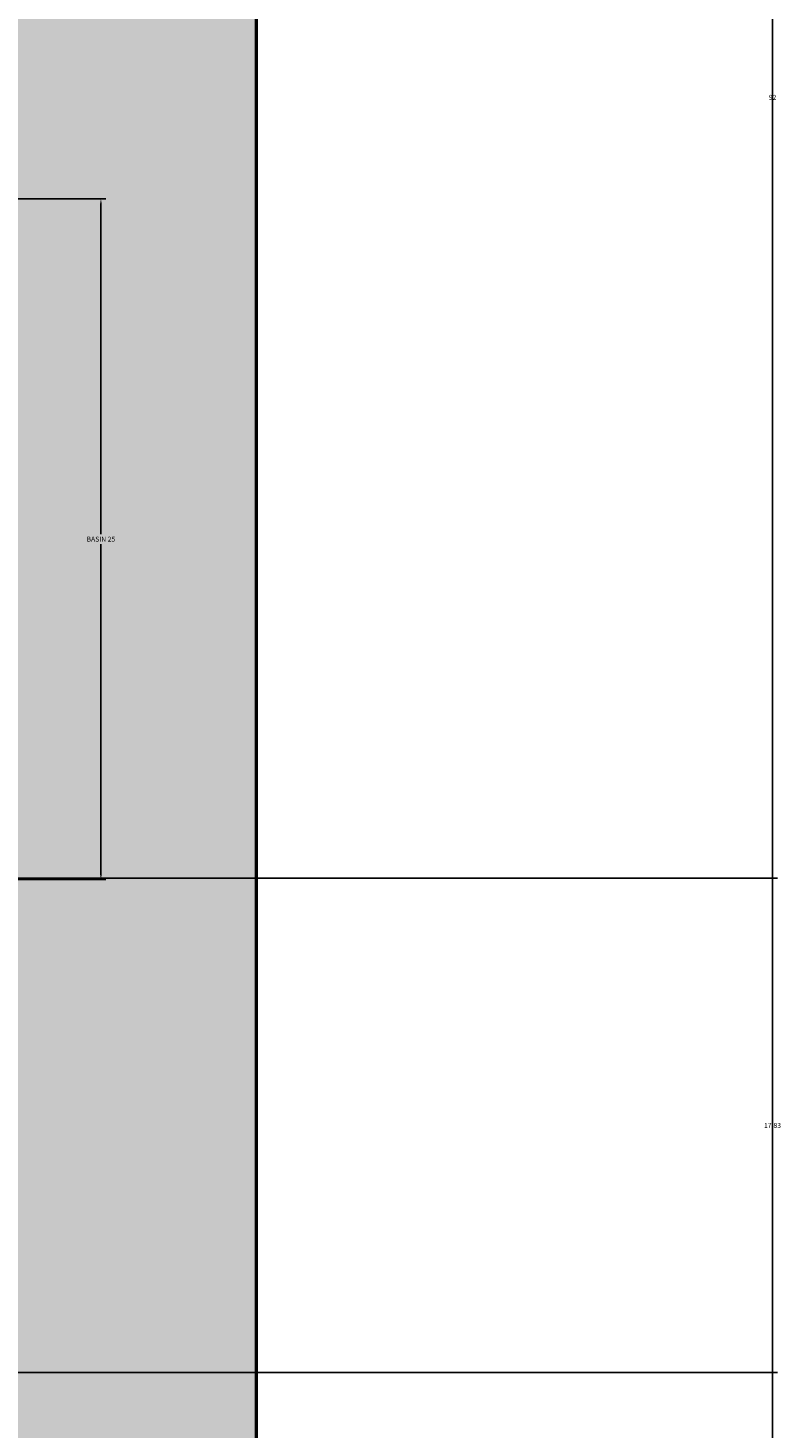
# Model space of a CAD drawing. Units: inches. Extents: x 2231 to 2461, y 2045 to 2455.
# Tile 85 of 95: x 2434 to 2461, y 2333 to 2383. Entities that reach past the tile are written whole.
import ezdxf

# ---------------------------------------------------------------- set-up
doc = ezdxf.new("R2010")
doc.units = ezdxf.units.IN
doc.layers.add('A-ANNO-DIMS', color=2, linetype='Continuous', lineweight=18)
doc.layers.add('A-WALL', color=7, linetype='Continuous', lineweight=50)
doc.layers.add('A-WALL-PATT', color=18, linetype='Continuous', lineweight=13, true_color=0x000000)
doc.styles.get("Standard").update_dxf_attribs({"font": 'arial.ttf'})
doc.dimstyles.get("Standard").update_dxf_attribs({"dimtxt": 0.18, "dimasz": 0.18, "dimexe": 0.18, "dimexo": 0.0625, "dimgap": 0.09, "dimtad": 0, "dimtih": 1, "dimtoh": 1, "dimdec": 4, "dimzin": 0, "dimdsep": 46, "dimtxsty": 'Standard', "dimcen": 0.09, "dimadec": 0, "dimazin": 0, "dimtfac": 1, "dimtdec": 4, "dimtofl": 0, "dimtmove": 0, "dimatfit": 3, "dimfxl": 1, "dimtolj": 1, "dimtzin": 0, "dimarcsym": 0})

# ---------------------------------------------------------------- blocks, each defined once
blk = doc.blocks.new('*D23')
at = {"layer": 'A-ANNO-DIMS', "color": 0, "lineweight": -2, "transparency": 16777216}
for p, q in [((2432.568, 2377.172), (2436.368, 2377.172)), ((2436.188, 2376.992), (2436.188, 2365.08)), ((2436.188, 2352.802), (2436.188, 2364.714)), ((2432.568, 2352.622), (2436.368, 2352.622))]:
    blk.add_line(p, q, dxfattribs=at)
at = {"layer": 'A-ANNO-DIMS', "color": 0, "transparency": 16777216}
for points in [[(2436.158, 2376.992), (2436.218, 2376.992), (2436.188, 2377.172)], [(2436.158, 2352.802), (2436.218, 2352.802), (2436.188, 2352.622)]]:
    blk.add_solid(points, dxfattribs=at)
at = {"layer": 'Defpoints', "color": 0, "transparency": 16777216}
for p in [(2432.506, 2377.172), (2432.506, 2352.622), (2436.188, 2352.622)]:
    blk.add_point(p, dxfattribs=at)
at = {"layer": 'A-ANNO-DIMS', "color": 0, "transparency": 16777216, "insert": (2436.188, 2364.897), "char_height": 0.18, "attachment_point": 5}
blk.add_mtext('\\A1;BASIN 25', dxfattribs=at)
blk = doc.blocks.new('*D34')
at = {"layer": 'A-ANNO-DIMS', "color": 0, "lineweight": -2, "transparency": 16777216}
for p, q in [((2441.856, 2435.833), (2460.606, 2435.833)), ((2460.426, 2435.653), (2460.426, 2250.015)), ((2460.426, 2064.013), (2460.426, 2249.651)), ((2441.856, 2063.833), (2460.606, 2063.833))]:
    blk.add_line(p, q, dxfattribs=at)
at = {"layer": 'A-ANNO-DIMS', "color": 0, "transparency": 16777216}
for points in [[(2460.396, 2435.653), (2460.456, 2435.653), (2460.426, 2435.833)], [(2460.396, 2064.013), (2460.456, 2064.013), (2460.426, 2063.833)]]:
    blk.add_solid(points, dxfattribs=at)
at = {"layer": 'Defpoints', "color": 0, "transparency": 16777216}
for p in [(2441.794, 2435.833), (2460.426, 2435.833), (2441.794, 2063.833)]:
    blk.add_point(p, dxfattribs=at)
at = {"layer": 'A-ANNO-DIMS', "color": 0, "transparency": 16777216, "insert": (2460.426, 2249.833), "char_height": 0.18, "attachment_point": 5}
blk.add_mtext('\\A1;372', dxfattribs=at)
blk = doc.blocks.new('*D38')
at = {"layer": 'A-ANNO-DIMS', "color": 0, "lineweight": -2, "transparency": 16777216}
for p, q in [((2432.856, 2426.833), (2460.606, 2426.833)), ((2460.426, 2426.653), (2460.426, 2381.015)), ((2460.426, 2335.013), (2460.426, 2380.651)), ((2432.856, 2334.833), (2460.606, 2334.833))]:
    blk.add_line(p, q, dxfattribs=at)
at = {"layer": 'A-ANNO-DIMS', "color": 0, "transparency": 16777216}
for points in [[(2460.396, 2426.653), (2460.456, 2426.653), (2460.426, 2426.833)], [(2460.396, 2335.013), (2460.456, 2335.013), (2460.426, 2334.833)]]:
    blk.add_solid(points, dxfattribs=at)
at = {"layer": 'Defpoints', "color": 0, "transparency": 16777216}
for p in [(2432.794, 2426.833), (2460.426, 2426.833), (2432.794, 2334.833)]:
    blk.add_point(p, dxfattribs=at)
at = {"layer": 'A-ANNO-DIMS', "color": 0, "transparency": 16777216, "insert": (2460.426, 2380.833), "char_height": 0.18, "attachment_point": 5}
blk.add_mtext('\\A1;92', dxfattribs=at)
blk = doc.blocks.new('*D76')
at = {"layer": 'A-ANNO-DIMS', "color": 0, "lineweight": -2, "transparency": 16777216}
for p, q in [((2422.106, 2352.663), (2460.606, 2352.663)), ((2460.426, 2352.483), (2460.426, 2343.93)), ((2460.426, 2335.013), (2460.426, 2343.566)), ((2432.856, 2334.833), (2460.606, 2334.833))]:
    blk.add_line(p, q, dxfattribs=at)
at = {"layer": 'A-ANNO-DIMS', "color": 0, "transparency": 16777216}
for points in [[(2460.396, 2352.483), (2460.456, 2352.483), (2460.426, 2352.663)], [(2460.396, 2335.013), (2460.456, 2335.013), (2460.426, 2334.833)]]:
    blk.add_solid(points, dxfattribs=at)
at = {"layer": 'Defpoints', "color": 0, "transparency": 16777216}
for p in [(2422.043, 2352.663), (2460.426, 2352.663), (2432.794, 2334.833)]:
    blk.add_point(p, dxfattribs=at)
at = {"layer": 'A-ANNO-DIMS', "color": 0, "transparency": 16777216, "insert": (2460.426, 2343.748), "char_height": 0.18, "attachment_point": 5}
blk.add_mtext('\\A1;17.83', dxfattribs=at)

msp = doc.modelspace()

# ---------------------------------------------------------------- hatches: boundary and pattern name
at = {"layer": 'A-WALL-PATT'}
h = msp.add_hatch(color=256, dxfattribs=at)
h.dxf.hatch_style = 1
h.paths.add_polyline_path([(2441.7935, 2269.1535), (2432.7935, 2269.1535), (2432.7935, 2186.8328), (2396.7935, 2186.8328), (2396.7935, 2286.8328), (2394.7935, 2286.8328), (2394.7935, 2186.8328), (2334.7935, 2186.8328), (2334.7935, 2182.8328), (2432.7935, 2182.8328), (2432.7935, 2072.8328), (2416.6639, 2072.8328), (2416.6639, 2063.8328), (2441.7935, 2063.8328)])
h.paths.add_polyline_path([(2368.6639, 2072.8328), (2367.04, 2072.8328), (2330.7942, 2072.8328), (2330.7397, 2063.8328), (2368.6639, 2063.8328)])
h.paths.add_polyline_path([(2300.7392, 2068.3328), (2300.7392, 2072.8328), (2298.7935, 2072.8328), (2294.7935, 2072.8328), (2258.7935, 2072.8328), (2258.7935, 2120.8328), (2294.7935, 2120.8328), (2298.7935, 2120.8328), (2298.7935, 2128.8328), (2294.7935, 2128.8328), (2294.7935, 2124.8328), (2258.7935, 2124.8328), (2258.7935, 2182.8328), (2294.7935, 2182.8328), (2294.7935, 2174.8328), (2298.7935, 2174.8328), (2298.7935, 2182.8328), (2304.7935, 2182.8328), (2304.7935, 2186.8328), (2258.7935, 2186.8328), (2258.7935, 2221.999), (2249.7935, 2221.999), (2249.7935, 2063.8328), (2300.7392, 2063.8328)])
h.paths.add_polyline_path([(2391.9338, 2435.8328), (2333.82, 2435.8328), (2333.82, 2426.8328), (2368.7935, 2426.8328), (2368.7935, 2374.9508), (2368.7935, 2370.8328), (2372.3935, 2370.8328), (2372.7935, 2370.8328), (2372.7935, 2426.8328), (2391.9338, 2426.8328)])
h.paths.add_polyline_path([(2441.7935, 2435.8328), (2415.9338, 2435.8328), (2415.9338, 2426.8328), (2432.7935, 2426.8328), (2432.7935, 2334.8328), (2372.7935, 2334.8328), (2372.7935, 2346.8328), (2368.7935, 2346.8328), (2368.7935, 2306.8328), (2360.7935, 2306.8328), (2360.7935, 2302.8328), (2368.7935, 2302.8328), (2372.7935, 2302.8328), (2372.7935, 2330.8328), (2432.7935, 2330.8328), (2432.7935, 2317.1535), (2441.7935, 2317.1535)])
h.paths.add_polyline_path([(2285.82, 2435.8328), (2249.7935, 2435.8328), (2249.7935, 2269.999), (2258.7935, 2269.999), (2258.7935, 2302.8328), (2318.8168, 2302.8328), (2330.7935, 2302.8328), (2330.7935, 2306.8328), (2258.7935, 2306.8328), (2258.7935, 2426.8328), (2285.82, 2426.8328)])

# ---------------------------------------------------------------- linework, layer by layer
at = {"layer": 'A-WALL'}
msp.add_lwpolyline([(2300.7392, 2063.8328), (2249.7935, 2063.8328), (2249.7935, 2435.8328), (2441.7935, 2435.8328), (2441.7935, 2063.8328), (2330.7397, 2063.8328)], dxfattribs=at)

# ---------------------------------------------------------------- dimensions: what is measured, and where the dimension line sits
at = {"layer": 'A-ANNO-DIMS'}
for base, p1, p2, override, picture, middle in [((2460.426, 2435.8328), (2441.7935, 2063.8328), (2441.7935, 2435.8328), {"dimdec": 0, "dimlfac": 1, "dimrnd": 0, "dimzin": 0, "dimdsep": 46, "dimlunit": 2}, '*D34', (2460.426, 2249.8328)), ((2460.426, 2426.8328), (2432.7935, 2334.8328), (2432.7935, 2426.8328), {"dimdec": 0, "dimlfac": 1, "dimrnd": 0, "dimzin": 0, "dimdsep": 46, "dimlunit": 2}, '*D38', (2460.426, 2380.8328)), ((2460.426, 2352.6633), (2432.7935, 2334.8328), (2422.0433, 2352.6633), {"dimdec": 2, "dimlfac": 1, "dimrnd": 0, "dimzin": 0, "dimdsep": 46, "dimlunit": 2}, '*D76', (2460.426, 2343.7481))]:
    dim = msp.add_linear_dim(base=base, p1=p1, p2=p2, angle=90, dimstyle='Standard', override=override, dxfattribs=at)
    dim.commit()
    dim.dimension.update_dxf_attribs({"geometry": picture, "text_midpoint": middle})
dim = msp.add_linear_dim(base=(2436.1885, 2352.6216), p1=(2432.5058, 2377.1725), p2=(2432.5058, 2352.6216), angle=270, text='BASIN <>', dimstyle='Standard', override={"dimdec": 0, "dimlfac": 1, "dimrnd": 0, "dimzin": 0, "dimdsep": 46, "dimlunit": 2}, dxfattribs=at)
dim.commit()
dim.dimension.update_dxf_attribs({"geometry": '*D23', "text_midpoint": (2436.1885, 2364.897)})

doc.saveas('drawing.dxf')
